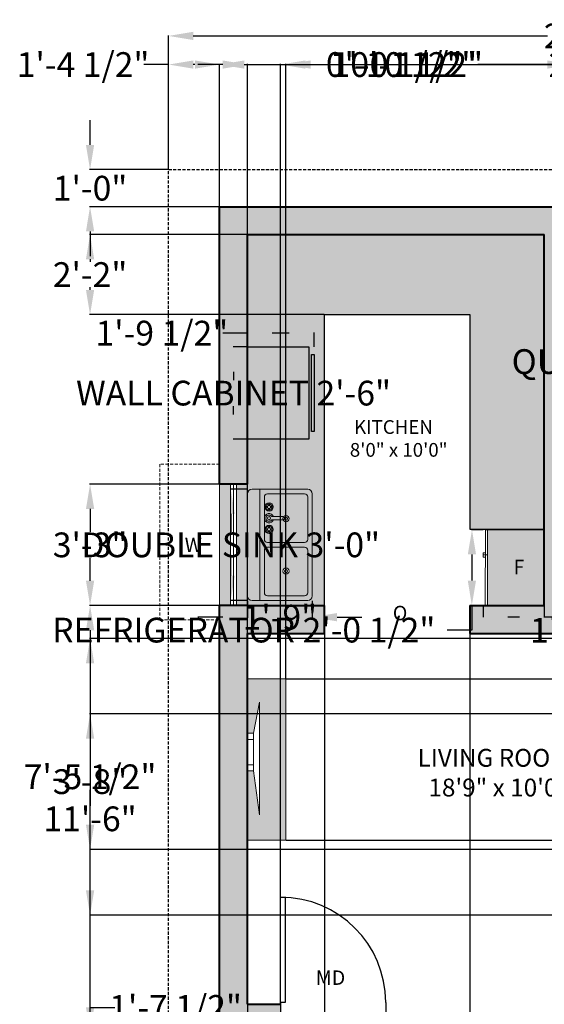
# Model space of a CAD drawing. Units: inches. Extents: x 277 to 728, y 649 to 1132.
# Tile 2 of 4: x 277 to 447, y 813 to 1132. Entities that reach past the tile are written whole.
import ezdxf

# ---------------------------------------------------------------- set-up
doc = ezdxf.new("R2010")
doc.units = ezdxf.units.IN
doc.header["$MEASUREMENT"] = 0
doc.linetypes.add('DASHEDX2', pattern=[1.5, 1, -0.5])
for name, color, linetype, lineweight in [('A-ANNO-DIMS', 2, 'Continuous', 18), ('A-ANNO-TEXT', 7, 'Continuous', 18), ('A-AREA-IDEN', 7, 'Continuous', 25), ('A-DOOR', 3, 'Continuous', 25), ('A-EQPM', 8, 'Continuous', 18), ('A-FLOR-CASE', 7, 'Continuous', 25), ('A-FLOR-FIXT', 8, 'Continuous', 18), ('A-FURN', 8, 'Continuous', 18), ('A-GLAZ', 4, 'Continuous', 18), ('A-GLAZ-OVHD', 8, 'DASHEDX2', 13), ('A-WALL', 7, 'Continuous', 40), ('A-WALL-PATT', 8, 'Continuous', 13), ('C-PROP', 7, 'DASHEDX2', 25)]:
    doc.layers.add(name, color=color, linetype=linetype, lineweight=lineweight)
for name, color, linetype, lineweight, true_color in [('A-EQPM-PATT', 30, 'Continuous', 9, 0xf7941d), ('A-FLOR-CASE-PATT', 18, 'Continuous', 9, 0x000000), ('A-FLOR-FIXT-PATT', 18, 'Continuous', 9, 0x000000), ('A-FURN-PATT', 9, 'Continuous', 9, 0xd6bdce), ('A-GLAZ-PATT', 144, 'Continuous', 13, 0x1e788f)]:
    doc.layers.add(name, color=color, linetype=linetype, lineweight=lineweight, true_color=true_color)
doc.styles.get("Standard").update_dxf_attribs({"font": 'arial.ttf'})
doc.dimstyles.get("Standard").update_dxf_attribs({"dimtxt": 8, "dimasz": 8, "dimexe": 0.18, "dimexo": 0.0625, "dimgap": 0.09, "dimtad": 0, "dimtih": 1, "dimtoh": 1, "dimdec": 0, "dimzin": 0, "dimdsep": 46, "dimlunit": 3, "dimtxsty": 'Standard', "dimcen": 0.09, "dimadec": 0, "dimazin": 0, "dimtfac": 1, "dimtdec": 0, "dimtofl": 0, "dimtmove": 0, "dimatfit": 3, "dimfxl": 1, "dimtolj": 1, "dimtzin": 0, "dimarcsym": 0})

# ---------------------------------------------------------------- blocks, each defined once
blk = doc.blocks.new('*U4')
for p, q in [((0, 0), (0, -6)), ((40, 0), (40, -6))]:
    blk.add_line(p, q)
blk.add_lwpolyline([(0, 0), (0, 40), (1.75, 40), (1.75, 0)], close=True)
blk.add_arc((0, 0), 40, 0, 90)
blk = doc.blocks.new('Faucet - Bathroom top')
for p, q in [((-4.107, 0.125), (-4.375, 0.125)), ((-3.75, 0.4788), (-3.75, 0.75)), ((-3.5, 0.482), (-3.5, 0.75)), ((-3.1461, 0.125), (-2.875, 0.125)), ((3.143, 0.125), (2.875, 0.125)), ((3.5, 0.4788), (3.5, 0.75)), ((3.75, 0.482), (3.75, 0.75)), ((4.1039, 0.125), (4.375, 0.125)), ((-4.1039, -0.125), (-4.375, -0.125)), ((-3.75, -0.4821), (-3.75, -0.75)), ((-3.5, -0.4789), (-3.5, -0.75)), ((-3.143, -0.125), (-2.875, -0.125)), ((-0.5, -0.8639), (-0.5, -4.5)), ((0.5, -4.5), (0.5, -0.8631)), ((3.1461, -0.125), (2.875, -0.125)), ((3.5, -0.4821), (3.5, -0.75)), ((3.75, -0.4789), (3.75, -0.75)), ((4.107, -0.125), (4.375, -0.125))]:
    blk.add_line(p, q)
for centre, radius in [((-3.625, 0), 1.375), ((-4.625, 0), 0.2795), ((-3.625, 0), 0.5), ((-3.625, 1), 0.2795), ((-2.625, 0), 0.2795), ((0, 0), 0.5), ((3.625, 0), 1.375), ((2.625, 0), 0.2795), ((3.625, 0), 0.5), ((3.625, 1), 0.2795), ((4.625, 0), 0.2795), ((-3.625, -1), 0.2795), ((3.625, -1), 0.2795)]:
    blk.add_circle(centre, radius)
for centre, radius, start, end in [((-3.625, 0), 1, 105.2407, 164.2093), ((-3.625, 0), 1, 16.44125, 74.07887), ((0, 0), 1.5, 289.6514, 250.3603), ((0, 0), 1, 300.3431, 239.7554), ((3.625, 0), 1, 106.12, 164.0884), ((3.625, 0), 1, 16.23422, 73.90469), ((-3.625, 0), 1, 196.2342, 253.9047), ((-3.625, 0), 1, 286.12, 344.0884), ((3.625, 0), 1, 196.4413, 254.0789), ((3.625, 0), 1, 285.2407, 344.2093), ((0, -4.5), 0.5, 180, 0)]:
    blk.add_arc(centre, radius, start, end)
blk = doc.blocks.new('Refrigerator-2 door - 36 in top')
for p, q in [((0, -26.999999), (36, -26.999999)), ((11, -27.999999), (11, -28.999999)), ((12, -26.999999), (12, -28.999999)), ((13, -28.999999), (13, -27.999999)), ((11, -28.999999), (13, -28.999999))]:
    blk.add_line(p, q)
blk.add_lwpolyline([(0, -27.999999), (0, 0), (36, 0), (36, -27.999999)], close=True)
blk = doc.blocks.new('Sink-double - 36 in top')
for p, q in [((-18, -4), (18, -4)), ((-0.75, -18.5), (-0.75, -6.5)), ((0.75, -6.5), (0.75, -18.5))]:
    blk.add_line(p, q)
for points in [[(-16.5, 0), (16.5, 0)], [(-18, -19.5), (-18, -1.5)], [(18, -1.5), (18, -19.5)], [(-15.5, -5.5), (-1.75, -5.5)], [(1.75, -5.5), (15.5, -5.5)], [(-16.5, -18.5), (-16.5, -6.5)], [(16.5, -6.5), (16.5, -18.5)], [(16.5, -21), (-16.5, -21)], [(-1.75, -19.5), (-15.5, -19.5)], [(15.5, -19.5), (1.75, -19.5)]]:
    blk.add_lwpolyline(points)
for centre, radius in [((-8.5, -12.5), 1), ((-8.5, -12.5), 0.5), ((8.5, -12.5), 1), ((8.5, -12.5), 0.5)]:
    blk.add_circle(centre, radius)
for centre, radius, start, end in [((-16.5, -1.5), 1.5, 90, 180), ((16.5, -1.5), 1.5, 0, 90), ((-15.5, -6.5), 1, 90, 180), ((-1.75, -6.5), 1, 0, 90), ((1.75, -6.5), 1, 90, 180), ((15.5, -6.5), 1, 0, 90), ((-15.5, -18.5), 1, 180, 270), ((-1.75, -18.5), 1, 270, 0), ((1.75, -18.5), 1, 180, 270), ((15.5, -18.5), 1, 270, 0), ((-16.5, -19.5), 1.5, 180, 270), ((16.5, -19.5), 1.5, 270, 0)]:
    blk.add_arc(centre, radius, start, end)
blk = doc.blocks.new('Wall Cabinet - 18 x 12 in side')
for points in [[(-12, -18), (-12, 0), (0, 0), (0, -18)], [(-13, -16.5), (-13, -1.5), (-12.5, -1.5), (-12.5, -16.5)]]:
    blk.add_lwpolyline(points, close=True)
blk = doc.blocks.new('*D20')
at = {"layer": 'A-ANNO-DIMS', "color": 0, "lineweight": -2, "transparency": 16777216}
for p, q in [((325.22, 1083.11), (325.22, 1126.48)), ((333.22, 1126.3), (447.82, 1126.3)), ((590.22, 1126.3), (475.62, 1126.3)), ((598.22, 1083.11), (598.22, 1126.48))]:
    blk.add_line(p, q, dxfattribs=at)
at = {"layer": 'A-ANNO-DIMS', "color": 0, "transparency": 16777216}
for points in [[(333.22, 1127.64), (333.22, 1124.97), (325.22, 1126.3)], [(590.22, 1127.64), (590.22, 1124.97), (598.22, 1126.3)]]:
    blk.add_solid(points, dxfattribs=at)
at = {"layer": 'Defpoints', "color": 0, "transparency": 16777216}
for p in [(598.22, 1126.3), (325.22, 1083.05), (598.22, 1083.05)]:
    blk.add_point(p, dxfattribs=at)
at = {"layer": 'A-ANNO-DIMS', "color": 0, "transparency": 16777216, "insert": (461.72, 1126.3), "char_height": 8, "attachment_point": 5}
blk.add_mtext('\\A1;22\'-9"', dxfattribs=at)
blk = doc.blocks.new('*D31')
at = {"layer": 'A-ANNO-DIMS', "color": 0, "lineweight": -2, "transparency": 16777216}
for p, q in [((426.99, 966.55), (423.2, 966.56)), ((423.37, 958.56), (423.35, 950.09)), ((426.95, 942.09), (423.16, 942.09)), ((423.34, 942.09), (423.32, 934.09)), ((423.32, 934.09), (415.32, 934.09))]:
    blk.add_line(p, q, dxfattribs=at)
at = {"layer": 'A-ANNO-DIMS', "color": 0, "transparency": 16777216}
for points in [[(422.04, 958.56), (424.7, 958.56), (423.38, 966.56)], [(422.02, 950.1), (424.69, 950.09), (423.34, 942.09)]]:
    blk.add_solid(points, dxfattribs=at)
at = {"layer": 'Defpoints', "color": 0, "transparency": 16777216}
for p in [(427.05, 966.55), (423.34, 942.09), (427.01, 942.09)]:
    blk.add_point(p, dxfattribs=at)
at = {"layer": 'A-ANNO-DIMS', "color": 0, "transparency": 16777216, "insert": (349.54, 934.09), "char_height": 8, "attachment_point": 5}
blk.add_mtext('\\A1;REFRIGERATOR 2\'-0 1/2"', dxfattribs=at)
blk = doc.blocks.new('*D32')
at = {"layer": 'A-ANNO-DIMS', "color": 0, "lineweight": -2, "transparency": 16777216}
for p, q in [((427.01, 942.02), (427, 938.24)), ((446.72, 941.99), (446.71, 938.2)), ((435, 938.4), (438.71, 938.4)), ((446.71, 938.38), (454.71, 938.37))]:
    blk.add_line(p, q, dxfattribs=at)
at = {"layer": 'A-ANNO-DIMS', "color": 0, "transparency": 16777216}
for points in [[(435, 939.74), (435, 937.07), (427, 938.42)], [(438.71, 939.73), (438.71, 937.06), (446.71, 938.38)]]:
    blk.add_solid(points, dxfattribs=at)
at = {"layer": 'Defpoints', "color": 0, "transparency": 16777216}
for p in [(427.01, 942.09), (446.72, 942.05), (446.71, 938.38)]:
    blk.add_point(p, dxfattribs=at)
at = {"layer": 'A-ANNO-DIMS', "color": 0, "transparency": 16777216, "insert": (474.38, 938.37), "char_height": 8, "attachment_point": 5}
blk.add_mtext('\\A1;1\'-7 1/2"', dxfattribs=at)
blk = doc.blocks.new('*D33')
at = {"layer": 'A-ANNO-DIMS', "color": 0, "lineweight": -2, "transparency": 16777216}
for p, q in [((350.66, 979.67), (345.14, 979.67)), ((345.32, 971.67), (345.32, 965.91)), ((345.32, 951.67), (345.32, 957.44)), ((350.66, 943.67), (345.14, 943.67))]:
    blk.add_line(p, q, dxfattribs=at)
at = {"layer": 'A-ANNO-DIMS', "color": 0, "transparency": 16777216}
for points in [[(343.99, 971.67), (346.65, 971.67), (345.32, 979.67)], [(343.99, 951.67), (346.65, 951.67), (345.32, 943.67)]]:
    blk.add_solid(points, dxfattribs=at)
at = {"layer": 'Defpoints', "color": 0, "transparency": 16777216}
for p in [(345.32, 979.67), (350.72, 979.67), (350.72, 943.67)]:
    blk.add_point(p, dxfattribs=at)
at = {"layer": 'A-ANNO-DIMS', "color": 0, "transparency": 16777216, "insert": (345.32, 961.67), "char_height": 8, "attachment_point": 5}
blk.add_mtext('\\A1;DOUBLE SINK 3\'-0"', dxfattribs=at)
blk = doc.blocks.new('*D34')
at = {"layer": 'A-ANNO-DIMS', "color": 0, "lineweight": -2, "transparency": 16777216}
for p, q in [((350.72, 943.61), (350.72, 938.09)), ((371.72, 943.61), (371.72, 938.09)), ((342.72, 938.27), (334.72, 938.27)), ((379.72, 938.27), (387.72, 938.27))]:
    blk.add_line(p, q, dxfattribs=at)
at = {"layer": 'A-ANNO-DIMS', "color": 0, "transparency": 16777216}
for points in [[(342.72, 939.61), (342.72, 936.94), (350.72, 938.27)], [(379.72, 939.61), (379.72, 936.94), (371.72, 938.27)]]:
    blk.add_solid(points, dxfattribs=at)
at = {"layer": 'Defpoints', "color": 0, "transparency": 16777216}
for p in [(350.72, 943.67), (371.72, 943.67), (350.72, 938.27)]:
    blk.add_point(p, dxfattribs=at)
at = {"layer": 'A-ANNO-DIMS', "color": 0, "transparency": 16777216, "insert": (361.22, 938.27), "char_height": 8, "attachment_point": 5}
blk.add_mtext('\\A1;1\'-9"', dxfattribs=at)
blk = doc.blocks.new('*D35')
at = {"layer": 'A-ANNO-DIMS', "color": 0, "lineweight": -2, "transparency": 16777216}
for p, q in [((350.66, 1025.68), (346.06, 1025.68)), ((346.24, 1017.68), (346.24, 1014.99)), ((346.24, 1003.84), (346.24, 1006.54)), ((350.66, 995.84), (346.06, 995.84))]:
    blk.add_line(p, q, dxfattribs=at)
at = {"layer": 'A-ANNO-DIMS', "color": 0, "transparency": 16777216}
for points in [[(344.91, 1017.68), (347.58, 1017.68), (346.24, 1025.68)], [(344.91, 1003.84), (347.58, 1003.84), (346.24, 995.84)]]:
    blk.add_solid(points, dxfattribs=at)
at = {"layer": 'Defpoints', "color": 0, "transparency": 16777216}
for p in [(350.72, 1025.68), (346.24, 995.84), (350.72, 995.84)]:
    blk.add_point(p, dxfattribs=at)
at = {"layer": 'A-ANNO-DIMS', "color": 0, "transparency": 16777216, "insert": (346.24, 1010.76), "char_height": 8, "attachment_point": 5}
blk.add_mtext('\\A1;WALL CABINET 2\'-6"', dxfattribs=at)
blk = doc.blocks.new('*D36')
at = {"layer": 'A-ANNO-DIMS', "color": 0, "lineweight": -2, "transparency": 16777216}
for p, q in [((350.72, 1030.16), (342.72, 1030.16)), ((350.72, 1025.75), (350.72, 1030.34)), ((364.27, 1030.16), (358.72, 1030.16)), ((372.27, 1025.75), (372.27, 1030.34))]:
    blk.add_line(p, q, dxfattribs=at)
at = {"layer": 'A-ANNO-DIMS', "color": 0, "transparency": 16777216}
for points in [[(358.72, 1031.49), (358.72, 1028.83), (350.72, 1030.16)], [(364.27, 1031.49), (364.27, 1028.83), (372.27, 1030.16)]]:
    blk.add_solid(points, dxfattribs=at)
at = {"layer": 'Defpoints', "color": 0, "transparency": 16777216}
for p in [(350.72, 1030.16), (350.72, 1025.68), (372.27, 1025.68)]:
    blk.add_point(p, dxfattribs=at)
at = {"layer": 'A-ANNO-DIMS', "color": 0, "transparency": 16777216, "insert": (323.05, 1030.16), "char_height": 8, "attachment_point": 5}
blk.add_mtext('\\A1;1\'-9 1/2"', dxfattribs=at)
blk = doc.blocks.new('*D37')
at = {"layer": 'A-ANNO-DIMS', "color": 0, "lineweight": -2, "transparency": 16777216}
for p, q in [((494.94, 1062.05), (482.49, 1062.05)), ((482.67, 1054.05), (482.67, 1025.43)), ((482.67, 987.86), (482.67, 1016.48)), ((494.94, 979.86), (482.49, 979.86))]:
    blk.add_line(p, q, dxfattribs=at)
at = {"layer": 'A-ANNO-DIMS', "color": 0, "transparency": 16777216}
for points in [[(481.34, 1054.05), (484, 1054.05), (482.67, 1062.05)], [(481.34, 987.86), (484, 987.86), (482.67, 979.86)]]:
    blk.add_solid(points, dxfattribs=at)
at = {"layer": 'Defpoints', "color": 0, "transparency": 16777216}
for p in [(482.67, 1062.05), (495, 1062.05), (495, 979.86)]:
    blk.add_point(p, dxfattribs=at)
at = {"layer": 'A-ANNO-DIMS', "color": 0, "transparency": 16777216, "insert": (482.67, 1020.96), "char_height": 8, "attachment_point": 5}
blk.add_mtext('\\A1;QUEEN BED 6\'-10"', dxfattribs=at)
blk = doc.blocks.new('*D40')
at = {"layer": 'A-ANNO-DIMS', "color": 0, "lineweight": -2, "transparency": 16777216}
for p, q in [((502.25, 961.37), (491.12, 961.37)), ((491.3, 953.37), (491.3, 950.05)), ((502.25, 942.05), (491.12, 942.05)), ((491.3, 942.05), (491.3, 934.05)), ((491.3, 934.05), (483.3, 934.05))]:
    blk.add_line(p, q, dxfattribs=at)
at = {"layer": 'A-ANNO-DIMS', "color": 0, "transparency": 16777216}
for points in [[(489.96, 953.37), (492.63, 953.37), (491.3, 961.37)], [(489.96, 950.05), (492.63, 950.05), (491.3, 942.05)]]:
    blk.add_solid(points, dxfattribs=at)
at = {"layer": 'Defpoints', "color": 0, "transparency": 16777216}
for p in [(502.31, 961.37), (491.3, 942.05), (502.31, 942.05)]:
    blk.add_point(p, dxfattribs=at)
at = {"layer": 'A-ANNO-DIMS', "color": 0, "transparency": 16777216, "insert": (463.63, 934.05), "char_height": 8, "attachment_point": 5}
blk.add_mtext('\\A1;1\'-7 1/2"', dxfattribs=at)
blk = doc.blocks.new('*D41')
at = {"layer": 'A-ANNO-DIMS', "color": 0, "lineweight": -2, "transparency": 16777216}
for p, q in [((505.29, 907.01), (299.63, 907.01)), ((299.81, 899.01), (299.81, 889.26)), ((299.81, 871.15), (299.81, 880.9)), ((505.29, 863.15), (299.63, 863.15))]:
    blk.add_line(p, q, dxfattribs=at)
at = {"layer": 'A-ANNO-DIMS', "color": 0, "transparency": 16777216}
for points in [[(298.48, 899.01), (301.15, 899.01), (299.81, 907.01)], [(298.48, 871.15), (301.15, 871.15), (299.81, 863.15)]]:
    blk.add_solid(points, dxfattribs=at)
at = {"layer": 'Defpoints', "color": 0, "transparency": 16777216}
for p in [(299.81, 907.01), (505.35, 907.01), (505.35, 863.15)]:
    blk.add_point(p, dxfattribs=at)
at = {"layer": 'A-ANNO-DIMS', "color": 0, "transparency": 16777216, "insert": (299.81, 885.08), "char_height": 8, "attachment_point": 5}
blk.add_mtext('\\A1;3\'-8"', dxfattribs=at)
blk = doc.blocks.new('*D43')
at = {"layer": 'A-ANNO-DIMS', "color": 0, "lineweight": -2, "transparency": 16777216}
for p, q in [((554.66, 931.4), (299.63, 931.4)), ((299.81, 923.4), (299.81, 890.87)), ((299.81, 849.9), (299.81, 882.42)), ((554.66, 841.9), (299.63, 841.9))]:
    blk.add_line(p, q, dxfattribs=at)
at = {"layer": 'A-ANNO-DIMS', "color": 0, "transparency": 16777216}
for points in [[(298.48, 923.4), (301.15, 923.4), (299.81, 931.4)], [(298.48, 849.9), (301.15, 849.9), (299.81, 841.9)]]:
    blk.add_solid(points, dxfattribs=at)
at = {"layer": 'Defpoints', "color": 0, "transparency": 16777216}
for p in [(299.81, 931.4), (554.72, 931.4), (554.72, 841.9)]:
    blk.add_point(p, dxfattribs=at)
at = {"layer": 'A-ANNO-DIMS', "color": 0, "transparency": 16777216, "insert": (299.81, 886.65), "char_height": 8, "attachment_point": 5}
blk.add_mtext('\\A1;7\'-5 1/2"', dxfattribs=at)
blk = doc.blocks.new('*D45')
at = {"layer": 'A-ANNO-DIMS', "color": 0, "lineweight": -2, "transparency": 16777216}
for p, q in [((363.23, 918.34), (626.51, 918.34)), ((626.33, 910.34), (626.33, 896.32)), ((626.33, 874.12), (626.33, 888.14)), ((363.23, 866.12), (626.51, 866.12))]:
    blk.add_line(p, q, dxfattribs=at)
at = {"layer": 'A-ANNO-DIMS', "color": 0, "transparency": 16777216}
for points in [[(625, 910.34), (627.67, 910.34), (626.33, 918.34)], [(625, 874.12), (627.67, 874.12), (626.33, 866.12)]]:
    blk.add_solid(points, dxfattribs=at)
at = {"layer": 'Defpoints', "color": 0, "transparency": 16777216}
for p in [(363.17, 918.34), (626.33, 918.34), (363.17, 866.12)]:
    blk.add_point(p, dxfattribs=at)
at = {"layer": 'A-ANNO-DIMS', "color": 0, "transparency": 16777216, "insert": (626.33, 892.23), "char_height": 8, "attachment_point": 5}
blk.add_mtext('\\A1;4\'-4"', dxfattribs=at)
blk = doc.blocks.new('*D46')
at = {"layer": 'A-ANNO-DIMS', "color": 0, "lineweight": -2, "transparency": 16777216}
for p, q in [((342.72, 1117.04), (334.72, 1117.04)), ((350.72, 918.4), (350.72, 1117.22)), ((363.17, 918.4), (363.17, 1117.22)), ((371.17, 1117.04), (379.17, 1117.04))]:
    blk.add_line(p, q, dxfattribs=at)
at = {"layer": 'A-ANNO-DIMS', "color": 0, "transparency": 16777216}
for points in [[(342.72, 1118.37), (342.72, 1115.71), (350.72, 1117.04)], [(371.17, 1118.37), (371.17, 1115.71), (363.17, 1117.04)]]:
    blk.add_solid(points, dxfattribs=at)
at = {"layer": 'Defpoints', "color": 0, "transparency": 16777216}
for p in [(363.17, 1117.04), (350.72, 918.34), (363.17, 918.34)]:
    blk.add_point(p, dxfattribs=at)
at = {"layer": 'A-ANNO-DIMS', "color": 0, "transparency": 16777216, "insert": (398.84, 1117.04), "char_height": 8, "attachment_point": 5}
blk.add_mtext('\\A1;1\'-0 1/2"', dxfattribs=at)
blk = doc.blocks.new('*D47')
at = {"layer": 'A-ANNO-DIMS', "color": 0, "lineweight": -2, "transparency": 16777216}
for p, q in [((341.72, 1071.11), (341.72, 1117.22)), ((349.72, 1117.04), (449.32, 1117.04)), ((576.72, 1117.04), (477.12, 1117.04)), ((584.72, 1071.11), (584.72, 1117.22))]:
    blk.add_line(p, q, dxfattribs=at)
at = {"layer": 'A-ANNO-DIMS', "color": 0, "transparency": 16777216}
for points in [[(349.72, 1118.37), (349.72, 1115.71), (341.72, 1117.04)], [(576.72, 1118.37), (576.72, 1115.71), (584.72, 1117.04)]]:
    blk.add_solid(points, dxfattribs=at)
at = {"layer": 'Defpoints', "color": 0, "transparency": 16777216}
for p in [(584.72, 1117.04), (341.72, 1071.05), (584.72, 1071.05)]:
    blk.add_point(p, dxfattribs=at)
at = {"layer": 'A-ANNO-DIMS', "color": 0, "transparency": 16777216, "insert": (463.22, 1117.04), "char_height": 8, "attachment_point": 5}
blk.add_mtext('\\A1;20\'-3"', dxfattribs=at)
blk = doc.blocks.new('*D49')
at = {"layer": 'A-ANNO-DIMS', "color": 0, "lineweight": -2, "transparency": 16777216}
for p, q in [((341.72, 1071.11), (341.72, 1117.22)), ((349.72, 1117.04), (379.69, 1117.04)), ((455.22, 1117.04), (425.24, 1117.04)), ((463.22, 1071.11), (463.22, 1117.22))]:
    blk.add_line(p, q, dxfattribs=at)
at = {"layer": 'A-ANNO-DIMS', "color": 0, "transparency": 16777216}
for points in [[(349.72, 1118.37), (349.72, 1115.71), (341.72, 1117.04)], [(455.22, 1118.37), (455.22, 1115.71), (463.22, 1117.04)]]:
    blk.add_solid(points, dxfattribs=at)
at = {"layer": 'Defpoints', "color": 0, "transparency": 16777216}
for p in [(463.22, 1117.04), (341.72, 1071.05), (463.22, 1071.05)]:
    blk.add_point(p, dxfattribs=at)
at = {"layer": 'A-ANNO-DIMS', "color": 0, "transparency": 16777216, "insert": (402.47, 1117.04), "char_height": 8, "attachment_point": 5}
blk.add_mtext('\\A1;10\'-1 1/2"', dxfattribs=at)
blk = doc.blocks.new('*D51')
at = {"layer": 'A-ANNO-DIMS', "color": 0, "lineweight": -2, "transparency": 16777216}
for p, q in [((341.66, 981.3), (299.63, 981.3)), ((299.81, 973.3), (299.81, 965.85)), ((299.81, 950.05), (299.81, 957.5)), ((341.66, 942.05), (299.63, 942.05))]:
    blk.add_line(p, q, dxfattribs=at)
at = {"layer": 'A-ANNO-DIMS', "color": 0, "transparency": 16777216}
for points in [[(298.48, 973.3), (301.15, 973.3), (299.81, 981.3)], [(298.48, 950.05), (301.15, 950.05), (299.81, 942.05)]]:
    blk.add_solid(points, dxfattribs=at)
at = {"layer": 'Defpoints', "color": 0, "transparency": 16777216}
for p in [(299.81, 981.3), (341.72, 981.3), (341.72, 942.05)]:
    blk.add_point(p, dxfattribs=at)
at = {"layer": 'A-ANNO-DIMS', "color": 0, "transparency": 16777216, "insert": (299.81, 961.67), "char_height": 8, "attachment_point": 5}
blk.add_mtext('\\A1;3\'-3"', dxfattribs=at)
blk = doc.blocks.new('*D52')
at = {"layer": 'A-ANNO-DIMS', "color": 0, "lineweight": -2, "transparency": 16777216}
for p, q in [((341.66, 942.05), (299.63, 942.05)), ((299.81, 934.05), (299.81, 877.23)), ((299.81, 812.05), (299.81, 868.88)), ((341.66, 804.05), (299.63, 804.05))]:
    blk.add_line(p, q, dxfattribs=at)
at = {"layer": 'A-ANNO-DIMS', "color": 0, "transparency": 16777216}
for points in [[(298.48, 934.05), (301.15, 934.05), (299.81, 942.05)], [(298.48, 812.05), (301.15, 812.05), (299.81, 804.05)]]:
    blk.add_solid(points, dxfattribs=at)
at = {"layer": 'Defpoints', "color": 0, "transparency": 16777216}
for p in [(299.81, 942.05), (341.72, 942.05), (341.72, 804.05)]:
    blk.add_point(p, dxfattribs=at)
at = {"layer": 'A-ANNO-DIMS', "color": 0, "transparency": 16777216, "insert": (299.81, 873.05), "char_height": 8, "attachment_point": 5}
blk.add_mtext('\\A1;11\'-6"', dxfattribs=at)
blk = doc.blocks.new('*D58')
at = {"layer": 'A-ANNO-DIMS', "color": 0, "lineweight": -2, "transparency": 16777216}
for p, q in [((342.72, 1117.04), (334.72, 1117.04)), ((350.72, 813.11), (350.72, 1117.22)), ((361.43, 813.11), (361.43, 1117.22)), ((369.43, 1117.04), (377.43, 1117.04))]:
    blk.add_line(p, q, dxfattribs=at)
at = {"layer": 'A-ANNO-DIMS', "color": 0, "transparency": 16777216}
for points in [[(342.72, 1118.37), (342.72, 1115.71), (350.72, 1117.04)], [(369.43, 1118.37), (369.43, 1115.71), (361.43, 1117.04)]]:
    blk.add_solid(points, dxfattribs=at)
at = {"layer": 'Defpoints', "color": 0, "transparency": 16777216}
for p in [(361.43, 1117.04), (350.72, 813.05), (361.43, 813.05)]:
    blk.add_point(p, dxfattribs=at)
at = {"layer": 'A-ANNO-DIMS', "color": 0, "transparency": 16777216, "insert": (400.59, 1117.04), "char_height": 8, "attachment_point": 5}
blk.add_mtext('\\A1;0\'-10 1/2"', dxfattribs=at)
blk = doc.blocks.new('*D63')
at = {"layer": 'A-ANNO-DIMS', "color": 0, "lineweight": -2, "transparency": 16777216}
for p, q in [((375.63, 932.99), (375.63, 661.09)), ((422.67, 932.99), (422.67, 661.09)), ((383.63, 661.27), (385.32, 661.27)), ((414.67, 661.27), (412.98, 661.27))]:
    blk.add_line(p, q, dxfattribs=at)
at = {"layer": 'A-ANNO-DIMS', "color": 0, "transparency": 16777216}
for points in [[(383.63, 662.6), (383.63, 659.93), (375.63, 661.27)], [(414.67, 662.6), (414.67, 659.93), (422.67, 661.27)]]:
    blk.add_solid(points, dxfattribs=at)
at = {"layer": 'Defpoints', "color": 0, "transparency": 16777216}
for p in [(375.63, 933.05), (422.67, 933.05), (422.67, 661.27)]:
    blk.add_point(p, dxfattribs=at)
at = {"layer": 'A-ANNO-DIMS', "color": 0, "transparency": 16777216, "insert": (399.15, 661.27), "char_height": 8, "attachment_point": 5}
blk.add_mtext('\\A1;3\'-11"', dxfattribs=at)
blk = doc.blocks.new('*D64')
at = {"layer": 'A-ANNO-DIMS', "color": 0, "lineweight": -2, "transparency": 16777216}
for p, q in [((299.81, 804.05), (299.81, 812.05)), ((299.81, 812.05), (307.81, 812.05)), ((540.6, 804.05), (299.63, 804.05)), ((299.81, 792.62), (299.81, 796.05)), ((535.66, 784.62), (299.63, 784.62))]:
    blk.add_line(p, q, dxfattribs=at)
at = {"layer": 'A-ANNO-DIMS', "color": 0, "transparency": 16777216}
for points in [[(298.48, 796.05), (301.15, 796.05), (299.81, 804.05)], [(298.48, 792.62), (301.15, 792.62), (299.81, 784.62)]]:
    blk.add_solid(points, dxfattribs=at)
at = {"layer": 'Defpoints', "color": 0, "transparency": 16777216}
for p in [(299.81, 804.05), (540.67, 804.05), (535.72, 784.62)]:
    blk.add_point(p, dxfattribs=at)
at = {"layer": 'A-ANNO-DIMS', "color": 0, "transparency": 16777216, "insert": (327.48, 812.05), "char_height": 8, "attachment_point": 5}
blk.add_mtext('\\A1;1\'-7 1/2"', dxfattribs=at)
blk = doc.blocks.new('*D65')
at = {"layer": 'A-ANNO-DIMS', "color": 0, "lineweight": -2, "transparency": 16777216}
for p, q in [((447.72, 1117.04), (439.72, 1117.04)), ((455.72, 942.11), (455.72, 1117.22)), ((462.81, 942.11), (462.81, 1117.22)), ((470.81, 1117.04), (478.81, 1117.04))]:
    blk.add_line(p, q, dxfattribs=at)
at = {"layer": 'A-ANNO-DIMS', "color": 0, "transparency": 16777216}
for points in [[(447.72, 1118.37), (447.72, 1115.71), (455.72, 1117.04)], [(470.81, 1118.37), (470.81, 1115.71), (462.81, 1117.04)]]:
    blk.add_solid(points, dxfattribs=at)
at = {"layer": 'Defpoints', "color": 0, "transparency": 16777216}
for p in [(462.81, 1117.04), (455.72, 942.05), (462.81, 942.05)]:
    blk.add_point(p, dxfattribs=at)
at = {"layer": 'A-ANNO-DIMS', "color": 0, "transparency": 16777216, "insert": (489.54, 1117.04), "char_height": 8, "attachment_point": 5}
blk.add_mtext('\\A1;0\'-7"', dxfattribs=at)
blk = doc.blocks.new('*D66')
at = {"layer": 'A-ANNO-DIMS', "color": 0, "lineweight": -2, "transparency": 16777216}
for p, q in [((350.72, 932.99), (350.72, 661.09)), ((375.63, 932.99), (375.63, 661.09)), ((342.72, 661.27), (334.72, 661.27)), ((383.63, 661.27), (391.63, 661.27))]:
    blk.add_line(p, q, dxfattribs=at)
at = {"layer": 'A-ANNO-DIMS', "color": 0, "transparency": 16777216}
for points in [[(342.72, 662.6), (342.72, 659.93), (350.72, 661.27)], [(383.63, 662.6), (383.63, 659.93), (375.63, 661.27)]]:
    blk.add_solid(points, dxfattribs=at)
at = {"layer": 'Defpoints', "color": 0, "transparency": 16777216}
for p in [(350.72, 933.05), (375.63, 933.05), (375.63, 661.27)]:
    blk.add_point(p, dxfattribs=at)
at = {"layer": 'A-ANNO-DIMS', "color": 0, "transparency": 16777216, "insert": (363.17, 661.27), "char_height": 8, "attachment_point": 5}
blk.add_mtext('\\A1;2\'-1"', dxfattribs=at)
blk = doc.blocks.new('*D67')
at = {"layer": 'A-ANNO-DIMS', "color": 0, "lineweight": -2, "transparency": 16777216}
for p, q in [((325.22, 1117.04), (317.22, 1117.04)), ((325.22, 1083.11), (325.22, 1117.22)), ((333.72, 1117.04), (333.22, 1117.04)), ((341.72, 1071.11), (341.72, 1117.22))]:
    blk.add_line(p, q, dxfattribs=at)
at = {"layer": 'A-ANNO-DIMS', "color": 0, "transparency": 16777216}
for points in [[(333.22, 1118.37), (333.22, 1115.71), (325.22, 1117.04)], [(333.72, 1118.37), (333.72, 1115.71), (341.72, 1117.04)]]:
    blk.add_solid(points, dxfattribs=at)
at = {"layer": 'Defpoints', "color": 0, "transparency": 16777216}
for p in [(325.22, 1117.04), (325.22, 1083.05), (341.72, 1071.05)]:
    blk.add_point(p, dxfattribs=at)
at = {"layer": 'A-ANNO-DIMS', "color": 0, "transparency": 16777216, "insert": (297.55, 1117.04), "char_height": 8, "attachment_point": 5}
blk.add_mtext('\\A1;1\'-4 1/2"', dxfattribs=at)
blk = doc.blocks.new('*D68')
at = {"layer": 'A-ANNO-DIMS', "color": 0, "lineweight": -2, "transparency": 16777216}
for p, q in [((299.81, 1091.05), (299.81, 1099.05)), ((325.16, 1083.05), (299.63, 1083.05)), ((341.66, 1071.05), (299.63, 1071.05)), ((299.81, 1063.05), (299.81, 1055.05))]:
    blk.add_line(p, q, dxfattribs=at)
at = {"layer": 'A-ANNO-DIMS', "color": 0, "transparency": 16777216}
for points in [[(298.48, 1091.05), (301.15, 1091.05), (299.81, 1083.05)], [(298.48, 1063.05), (301.15, 1063.05), (299.81, 1071.05)]]:
    blk.add_solid(points, dxfattribs=at)
at = {"layer": 'Defpoints', "color": 0, "transparency": 16777216}
for p in [(299.81, 1083.05), (325.22, 1083.05), (341.72, 1071.05)]:
    blk.add_point(p, dxfattribs=at)
at = {"layer": 'A-ANNO-DIMS', "color": 0, "transparency": 16777216, "insert": (299.81, 1077.05), "char_height": 8, "attachment_point": 5}
blk.add_mtext('\\A1;1\'-0"', dxfattribs=at)
blk = doc.blocks.new('*D74')
at = {"layer": 'A-ANNO-DIMS', "color": 0, "lineweight": -2, "transparency": 16777216}
for p, q in [((350.66, 1062.05), (299.63, 1062.05)), ((299.81, 1054.05), (299.81, 1053.21)), ((299.81, 1044.15), (299.81, 1045)), ((375.57, 1036.15), (299.63, 1036.15))]:
    blk.add_line(p, q, dxfattribs=at)
at = {"layer": 'A-ANNO-DIMS', "color": 0, "transparency": 16777216}
for points in [[(298.48, 1054.05), (301.15, 1054.05), (299.81, 1062.05)], [(298.48, 1044.15), (301.15, 1044.15), (299.81, 1036.15)]]:
    blk.add_solid(points, dxfattribs=at)
at = {"layer": 'Defpoints', "color": 0, "transparency": 16777216}
for p in [(299.81, 1062.05), (350.72, 1062.05), (375.63, 1036.15)]:
    blk.add_point(p, dxfattribs=at)
at = {"layer": 'A-ANNO-DIMS', "color": 0, "transparency": 16777216, "insert": (299.81, 1049.1), "char_height": 8, "attachment_point": 5}
blk.add_mtext('\\A1;2\'-2"', dxfattribs=at)

msp = doc.modelspace()

# ---------------------------------------------------------------- hatches: boundary and pattern name
at = {"layer": 'A-EQPM-PATT'}
h = msp.add_hatch(color=256, dxfattribs=at)
h.dxf.hatch_style = 1
h.paths.add_polyline_path([(428.37, 942.08), (446.72, 942.05), (446.72, 966.52), (428.41, 966.55)])
h.paths.add_polyline_path([(435.13, 949.62), (441.43, 949.62), (441.43, 959.23), (435.13, 959.23)], flags=24)
at = {"layer": 'A-FLOR-CASE-PATT'}
h = msp.add_hatch(color=256, dxfattribs=at)
h.dxf.hatch_style = 1
h.paths.add_polyline_path([(350.72, 1025.68), (370.61, 1025.68), (370.61, 995.84), (350.72, 995.84), (350.72, 981.3), (350.72, 978.17, -0.414214), (352.22, 979.67), (370.22, 979.67, -0.414214), (371.72, 978.17), (371.72, 945.17, -0.414214), (370.22, 943.67), (352.22, 943.67, -0.414214), (350.72, 945.17), (350.72, 942.05), (375.63, 942.05), (375.63, 1036.15), (422.67, 1036.15), (422.67, 966.74), (446.72, 966.74), (446.72, 1062.05), (350.72, 1062.05)])
h.paths.add_polyline_path([(370.61, 1025.68), (370.61, 995.84), (350.72, 995.84), (350.72, 1025.68)], flags=17)
at = {"layer": 'A-FLOR-FIXT-PATT'}
h = msp.add_hatch(color=256, dxfattribs=at)
h.dxf.hatch_style = 1
h.paths.add_polyline_path([(350.72, 945.17, 0.414214), (352.22, 943.67), (354.72, 943.67), (354.72, 979.67), (352.22, 979.67, 0.414214), (350.72, 978.17)])
h = msp.add_hatch(color=256, dxfattribs=at)
h.dxf.hatch_style = 1
h.paths.add_polyline_path([(356.22, 946.17, 0.414214), (357.22, 945.17), (369.22, 945.17, 0.414214), (370.22, 946.17), (370.22, 959.92, 0.414214), (369.22, 960.92), (357.22, 960.92, 0.414214), (356.22, 959.92)], flags=16)
h.paths.add_polyline_path([(354.72, 943.67), (370.22, 943.67, 0.414214), (371.72, 945.17), (371.72, 978.17, 0.414214), (370.22, 979.67), (354.72, 979.67)])
h.paths.add_polyline_path([(362.22, 953.17, -1), (364.22, 953.17, -1)], flags=0)
h = msp.add_hatch(color=256, dxfattribs=at)
h.dxf.hatch_style = 1
h.paths.add_polyline_path([(369.22, 945.17, 0.414214), (370.22, 946.17), (370.22, 959.92, 0.414214), (369.22, 960.92), (357.22, 960.92, 0.414214), (356.22, 959.92), (356.22, 946.17, 0.414214), (357.22, 945.17)], flags=16)
h.paths.add_polyline_path([(370.22, 943.67, 0.414214), (371.72, 945.17), (371.72, 978.17, 0.414214), (370.22, 979.67), (354.72, 979.67), (354.72, 943.67)])
h.paths.add_polyline_path([(362.22, 953.17, -1), (364.22, 953.17, -1)], flags=0)
h = msp.add_hatch(color=256, dxfattribs=at)
h.dxf.hatch_style = 1
h.paths.add_polyline_path([(356.22, 946.17, 0.414214), (357.22, 945.17), (369.22, 945.17, 0.414214), (370.22, 946.17), (370.22, 959.92, 0.414214), (369.22, 960.92), (357.22, 960.92, 0.414214), (356.22, 959.92)], flags=16)
h.paths.add_polyline_path([(364.22, 953.17, -1), (362.22, 953.17, -1)], flags=0)
h.paths.add_polyline_path([(354.72, 943.67), (370.22, 943.67, 0.414214), (371.72, 945.17), (371.72, 978.17, 0.414214), (370.22, 979.67), (354.72, 979.67)])
h = msp.add_hatch(color=256, dxfattribs=at)
h.dxf.hatch_style = 1
h.paths.add_polyline_path([(362.22, 953.17, 1), (364.22, 953.17, 1)], flags=16)
h.paths.add_polyline_path([(362.72, 953.17, -1), (363.72, 953.17, -1)], flags=0)
h.paths.add_polyline_path([(370.22, 959.92, 0.414214), (369.22, 960.92), (357.22, 960.92, 0.414214), (356.22, 959.92), (356.22, 946.17, 0.414214), (357.22, 945.17), (369.22, 945.17, 0.414214), (370.22, 946.17)])
at = {"layer": 'A-FURN-PATT'}
h = msp.add_hatch(color=256, dxfattribs=at)
h.dxf.hatch_style = 1
h.paths.add_polyline_path([(354.62, 874.37), (352.72, 888.53), (350.72, 888.53), (350.72, 866.12), (363.17, 866.12), (363.17, 918.34), (350.72, 918.34), (350.72, 900.76), (352.72, 900.76), (354.62, 910.78)])
at = {"layer": 'A-GLAZ-PATT'}
h = msp.add_hatch(color=256, dxfattribs=at)
h.dxf.hatch_style = 1
h.paths.add_polyline_path([(345.22, 981.3), (341.72, 981.3), (341.72, 942.05), (345.22, 942.05)])
h = msp.add_hatch(color=256, dxfattribs=at)
h.dxf.hatch_style = 1
h.paths.add_polyline_path([(350.72, 981.3), (347.22, 981.3), (347.22, 942.05), (350.72, 942.05)])
at = {"layer": 'A-WALL-PATT'}
h = msp.add_hatch(color=256, dxfattribs=at)
h.dxf.hatch_style = 1
h.paths.add_polyline_path([(446.72, 942.05), (422.67, 942.05), (422.67, 933.05), (462.81, 933.05), (462.81, 942.05), (455.72, 942.05), (455.72, 1062.05), (463.22, 1062.05), (463.22, 1071.05), (341.72, 1071.05), (341.72, 981.3), (350.72, 981.3), (350.72, 1062.05), (446.72, 1062.05)])
h = msp.add_hatch(color=256, dxfattribs=at)
h.dxf.hatch_style = 1
h.paths.add_polyline_path([(361.43, 804.05), (361.43, 813.05), (350.72, 813.05), (350.72, 933.05), (375.63, 933.05), (375.63, 942.05), (350.72, 942.05), (341.72, 942.05), (341.72, 804.05)])

# ---------------------------------------------------------------- linework, layer by layer
at = {"layer": 'A-FLOR-CASE'}
for p, q in [((375.63, 942.05), (375.63, 1036.15)), ((375.63, 1036.15), (422.67, 1036.15)), ((422.67, 1036.15), (422.67, 966.74)), ((422.67, 966.74), (446.72, 966.74))]:
    msp.add_line(p, q, dxfattribs=at)
at = {"layer": 'A-FURN'}
for p, q in [((350.72, 918.34), (363.17, 918.34)), ((363.17, 918.34), (363.17, 866.12)), ((352.72, 900.76), (354.62, 910.78)), ((354.62, 910.78), (354.62, 874.37)), ((352.72, 900.76), (350.72, 900.76)), ((350.72, 900.76), (350.72, 898.76)), ((350.72, 898.76), (352.72, 898.76)), ((352.72, 888.53), (352.72, 900.76)), ((350.72, 888.53), (350.72, 890.53)), ((350.72, 890.53), (352.72, 890.53)), ((352.72, 888.53), (350.72, 888.53)), ((354.62, 874.37), (352.72, 888.53)), ((363.17, 866.12), (350.72, 866.12))]:
    msp.add_line(p, q, dxfattribs=at)
at = {"layer": 'A-GLAZ'}
for p, q in [((341.72, 981.3), (341.72, 942.05)), ((345.22, 981.3), (345.22, 942.05)), ((346.22, 981.3), (346.22, 942.05)), ((347.22, 981.3), (347.22, 942.05)), ((350.72, 981.3), (350.72, 942.05))]:
    msp.add_line(p, q, dxfattribs=at)
at = {"layer": 'A-GLAZ-OVHD'}
for p, q in [((341.72, 987.81), (322.41, 987.81)), ((322.41, 987.81), (322.41, 937.37)), ((322.41, 937.37), (341.72, 937.37))]:
    msp.add_line(p, q, dxfattribs=at)
at = {"layer": 'A-WALL'}
for p, q in [((341.72, 1071.05), (463.22, 1071.05)), ((341.72, 981.3), (341.72, 1071.05)), ((350.72, 1062.05), (446.72, 1062.05)), ((350.72, 981.3), (350.72, 1062.05)), ((446.72, 942.05), (446.72, 1062.05)), ((350.72, 981.3), (341.72, 981.3)), ((341.72, 723.05), (341.72, 942.05)), ((350.72, 942.05), (341.72, 942.05)), ((350.72, 942.05), (375.63, 942.05)), ((375.63, 933.05), (375.63, 942.05)), ((422.67, 942.05), (422.67, 933.05)), ((422.67, 942.05), (446.72, 942.05)), ((350.72, 813.05), (350.72, 933.05)), ((350.72, 933.05), (375.63, 933.05)), ((422.67, 933.05), (462.81, 933.05)), ((350.72, 813.05), (361.43, 813.05))]:
    msp.add_line(p, q, dxfattribs=at)
at = {"layer": 'C-PROP'}
for p, q in [((325.22, 723.05), (325.22, 1083.05)), ((325.22, 1083.05), (598.22, 1083.05))]:
    msp.add_line(p, q, dxfattribs=at)

# ---------------------------------------------------------------- block references
at = {"layer": 'A-DOOR', "xscale": 0.8508858402266032, "yscale": 0.8508858402266032, "zscale": 0.8508858402266032}
msp.add_blockref('*U4', (361.43, 813.66), dxfattribs=at)
at = {"layer": 'A-EQPM', "xscale": 0.6796353353316987, "yscale": 0.6796353353316987, "zscale": 0.6796353353316987, "rotation": 269.8953229012981}
msp.add_blockref('Refrigerator-2 door - 36 in top', (446.76, 966.52), dxfattribs=at)
at = {"layer": 'A-FLOR-CASE', "xscale": 1.65791062378445, "yscale": 1.65791062378445, "zscale": 1.65791062378445, "rotation": 180}
msp.add_blockref('Wall Cabinet - 18 x 12 in side', (350.72, 995.84), dxfattribs=at)
at = {"layer": 'A-FLOR-FIXT', "rotation": 90}
for name, p in [('Sink-double - 36 in top', (350.72, 961.67)), ('Faucet - Bathroom top', (357.72, 970.3))]:
    msp.add_blockref(name, p, dxfattribs=at)

# ---------------------------------------------------------------- texts
at = {"layer": 'A-ANNO-TEXT', "char_height": 4.66, "attachment_point": 1}
for s, insert in [('W', (330.44, 963.99)), ('F', (436.83, 956.83)), ('O', (397.76, 941.95)), ('MD', (372.85, 824))]:
    msp.add_mtext_dynamic_manual_height_columns(s, width=6.3557, gutter_width=23.3, heights=[0], dxfattribs=dict(at, insert=insert))
at = {"layer": 'A-AREA-IDEN', "attachment_point": 1}
for s, width, gutter_width, insert, char_height in [(' KITCHEN\\P8\'0" x 10\'0"', 54.6109, 22.18, (383.86, 1002.01), 4.4364), ('LIVING ROOM\\P  18\'9" x 10\'0"', 70.9765, 28.83, (405.77, 895.67), 5.7659)]:
    msp.add_mtext_dynamic_manual_height_columns(s, width=width, gutter_width=gutter_width, heights=[0], dxfattribs=dict(at, insert=insert, char_height=char_height))

# ---------------------------------------------------------------- dimensions: what is measured, and where the dimension line sits
at = {"layer": 'A-ANNO-DIMS'}
for base, p1, p2, override, picture, middle in [((598.22, 1126.3), (325.22, 1083.05), (598.22, 1083.05), {"dimclrd": 0, "dimclre": 0, "dimclrt": 0}, '*D20', (461.72, 1126.3)), ((325.22, 1117.04), (341.72, 1071.05), (325.22, 1083.05), {"dimdec": 1, "dimlfac": 1, "dimrnd": 0, "dimzin": 1, "dimdsep": 46, "dimlunit": 4, "dimfrac": 2}, '*D67', (297.55, 1117.04)), ((363.1693, 1117.0403), (350.7185, 918.3365), (363.1693, 918.3365), {"dimdec": 1, "dimlfac": 1, "dimrnd": 0, "dimzin": 1, "dimdsep": 46, "dimlunit": 4, "dimfrac": 2}, '*D46', (398.8364, 1117.0403)), ((361.43, 1117.04), (350.72, 813.05), (361.43, 813.05), {"dimdec": 1, "dimlfac": 1, "dimrnd": 0, "dimzin": 1, "dimdsep": 46, "dimlunit": 4, "dimfrac": 2}, '*D58', (400.59, 1117.04)), ((463.22, 1117.04), (341.72, 1071.05), (463.22, 1071.05), {"dimdec": 1, "dimlfac": 1, "dimrnd": 0, "dimzin": 1, "dimdsep": 46, "dimlunit": 4, "dimfrac": 2}, '*D49', (402.47, 1117.04)), ((584.72, 1117.04), (341.72, 1071.05), (584.72, 1071.05), {"dimdec": 1, "dimlfac": 1, "dimrnd": 0, "dimzin": 1, "dimdsep": 46, "dimlunit": 4, "dimfrac": 2}, '*D47', (463.22, 1117.04)), ((462.81, 1117.04), (455.72, 942.05), (462.81, 942.05), {"dimdec": 1, "dimlfac": 1, "dimrnd": 0, "dimzin": 1, "dimdsep": 46, "dimlunit": 4, "dimfrac": 2}, '*D65', (489.54, 1117.04)), ((375.63, 661.27), (350.72, 933.05), (375.63, 933.05), {"dimdec": 1, "dimlfac": 1, "dimrnd": 0, "dimzin": 1, "dimdsep": 46, "dimlunit": 4, "dimfrac": 2}, '*D66', (363.17, 661.27)), ((422.67, 661.27), (375.63, 933.05), (422.67, 933.05), {"dimdec": 1, "dimlfac": 1, "dimrnd": 0, "dimzin": 1, "dimdsep": 46, "dimlunit": 4, "dimfrac": 2}, '*D63', (399.15, 661.27))]:
    dim = msp.add_linear_dim(base=base, p1=p1, p2=p2, dimstyle='Standard', override=override, dxfattribs=at)
    dim.commit()
    dim.dimension.update_dxf_attribs({"geometry": picture, "text_midpoint": middle})
for base, p1, p2, angle, picture, middle in [((299.81, 1083.05), (341.72, 1071.05), (325.22, 1083.05), 90, '*D68', (299.81, 1077.05)), ((299.81, 1062.05), (375.63, 1036.15), (350.72, 1062.05), 90, '*D74', (299.81, 1049.1)), ((350.7185, 1030.1601), (372.2713, 1025.6837), (350.7185, 1025.6837), 180, '*D36', (323.0514, 1030.1601)), ((299.8136, 981.2986), (341.7185, 942.0508), (341.7185, 981.2986), 90, '*D51', (299.8136, 961.6747)), ((491.3, 942.05), (502.31, 961.37), (502.31, 942.05), 270, '*D40', (463.63, 934.05)), ((446.71, 938.38), (427.01, 942.09), (446.72, 942.05), 359.8953, '*D32', (474.38, 938.37)), ((350.72, 938.27), (371.72, 943.67), (350.72, 943.67), 180, '*D34', (361.22, 938.27)), ((299.81, 942.05), (341.72, 804.05), (341.72, 942.05), 90, '*D52', (299.81, 873.05)), ((299.81, 931.4), (554.72, 841.9), (554.72, 931.4), 90, '*D43', (299.81, 886.65)), ((626.33, 918.34), (363.17, 866.12), (363.17, 918.34), 90, '*D45', (626.33, 892.23)), ((299.81, 907.01), (505.35, 863.15), (505.35, 907.01), 90, '*D41', (299.81, 885.08)), ((299.81, 804.05), (535.72, 784.62), (540.67, 804.05), 90, '*D64', (327.48, 812.05))]:
    dim = msp.add_linear_dim(base=base, p1=p1, p2=p2, angle=angle, dimstyle='Standard', override={"dimdec": 1, "dimlfac": 1, "dimrnd": 0, "dimzin": 1, "dimdsep": 46, "dimlunit": 4, "dimfrac": 2}, dxfattribs=at)
    dim.commit()
    dim.dimension.update_dxf_attribs({"geometry": picture, "text_midpoint": middle})
for base, p1, p2, angle, text, picture, middle in [((482.67, 1062.05), (495, 979.86), (495, 1062.05), 90, 'QUEEN BED <>', '*D37', (482.67, 1020.96)), ((346.24, 995.84), (350.72, 1025.68), (350.72, 995.84), 270, 'WALL CABINET <>', '*D35', (346.24, 1010.76)), ((345.32, 979.67), (350.72, 943.67), (350.72, 979.67), 90, 'DOUBLE SINK <>', '*D33', (345.32, 961.67)), ((423.34, 942.09), (427.05, 966.55), (427.01, 942.09), 269.8953, 'REFRIGERATOR <>', '*D31', (349.54, 934.09))]:
    dim = msp.add_linear_dim(base=base, p1=p1, p2=p2, angle=angle, text=text, dimstyle='Standard', override={"dimdec": 1, "dimlfac": 1, "dimrnd": 0, "dimzin": 1, "dimdsep": 46, "dimlunit": 4, "dimfrac": 2}, dxfattribs=at)
    dim.commit()
    dim.dimension.update_dxf_attribs({"geometry": picture, "text_midpoint": middle})

doc.saveas('drawing.dxf')
